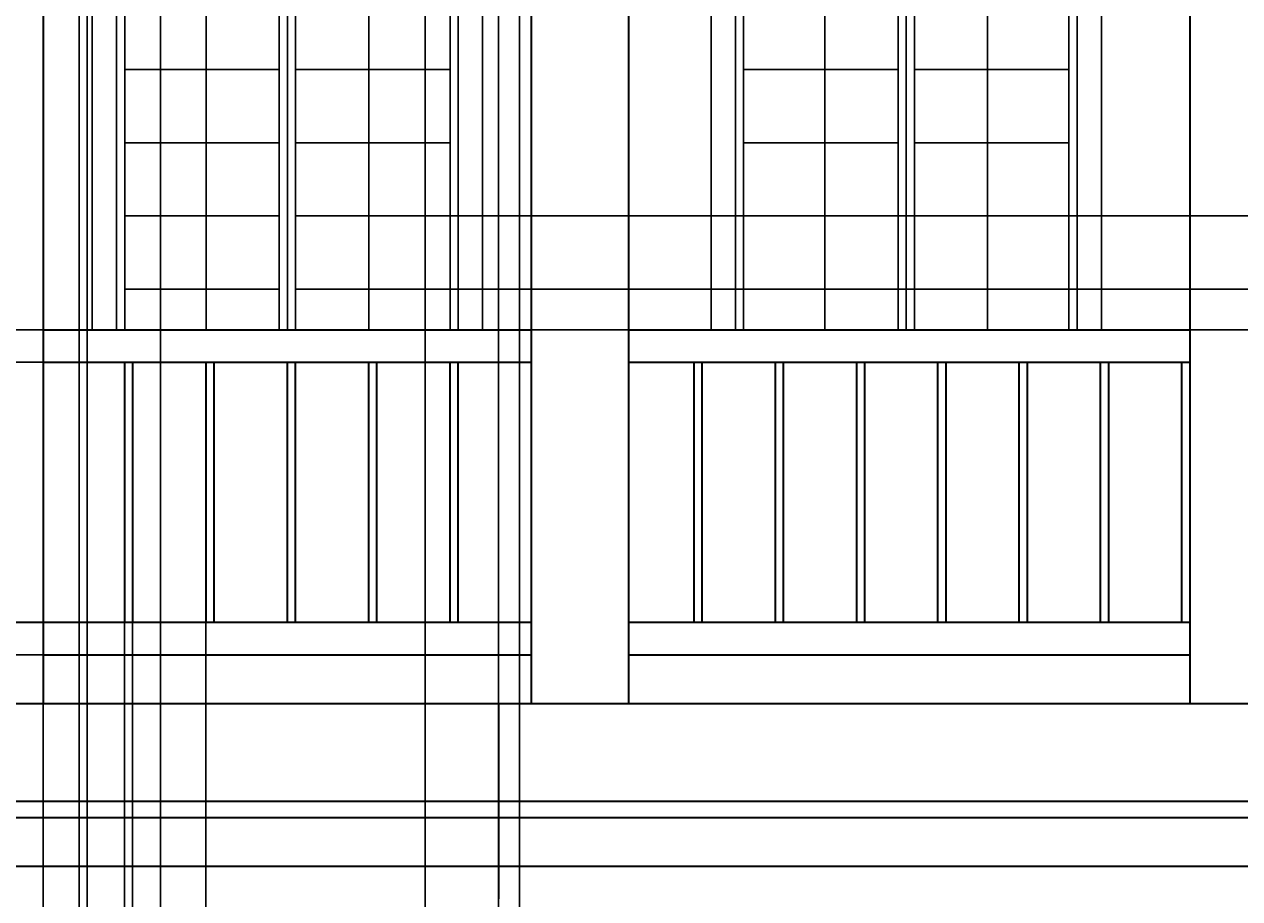
# Model space of a CAD drawing. Units: inches. Extents: x 2154 to 2740, y 571 to 1084.
# Tile 3 of 13: x 2235 to 2384, y 754 to 861. Entities that reach past the tile are written whole.
import ezdxf

# ---------------------------------------------------------------- set-up
doc = ezdxf.new("R2010")
doc.units = ezdxf.units.IN
for name, color, linetype, lineweight in [('A-ANNO-DIMS', 2, 'Continuous', 18), ('A-ELEV', 7, 'Continuous', 35), ('A-GLAZ', 4, 'Continuous', 25)]:
    doc.layers.add(name, color=color, linetype=linetype, lineweight=lineweight)
doc.styles.get("Standard").update_dxf_attribs({"font": 'arial.ttf'})
doc.dimstyles.get("Standard").update_dxf_attribs({"dimtxt": 0.18, "dimasz": 0.18, "dimexe": 0.18, "dimexo": 0.0625, "dimgap": 0.09, "dimtad": 0, "dimtih": 1, "dimtoh": 1, "dimdec": 4, "dimzin": 0, "dimdsep": 46, "dimtxsty": 'Standard', "dimcen": 0.09, "dimadec": 0, "dimazin": 0, "dimtfac": 1, "dimtdec": 4, "dimtofl": 0, "dimtmove": 0, "dimatfit": 3, "dimfxl": 1, "dimtolj": 1, "dimtzin": 0, "dimarcsym": 0})

# ---------------------------------------------------------------- blocks, each defined once
blk = doc.blocks.new('WIN-ELEV-1200')
for p, q in [((0, 50), (48, 50)), ((0, 0), (0, 50)), ((48, 0), (48, 50)), ((3, 0), (3, 47)), ((3, 47), (45, 47)), ((45, 0), (45, 47)), ((4, 46), (44, 46)), ((4, 0), (4, 46)), ((14, 0), (14, 46)), ((23, 0), (23, 46)), ((24, 0), (24, 46)), ((25, 0), (25, 46)), ((34, 0), (34, 46)), ((44, 0), (44, 46)), ((4, 41), (23, 41)), ((25, 41), (44, 41)), ((4, 32), (23, 32)), ((25, 32), (44, 32)), ((4, 23), (23, 23)), ((25, 23), (44, 23)), ((4, 14), (23, 14)), ((25, 14), (44, 14)), ((4, 5), (23, 5)), ((25, 5), (44, 5))]:
    blk.add_line(p, q)
blk = doc.blocks.new('*D10')
at = {"layer": 'A-ANNO-DIMS', "color": 0, "lineweight": -2, "transparency": 16777216}
for p, q in [((2447.14, 1057.01), (2154.18, 1057.01)), ((2154.36, 1056.83), (2154.36, 827.45)), ((2154.36, 597.71), (2154.36, 827.09)), ((2181.14, 597.53), (2154.18, 597.53))]:
    blk.add_line(p, q, dxfattribs=at)
at = {"layer": 'A-ANNO-DIMS', "color": 0, "transparency": 16777216}
for points in [[(2154.33, 1056.83), (2154.39, 1056.83), (2154.36, 1057.01)], [(2154.33, 597.71), (2154.39, 597.71), (2154.36, 597.53)]]:
    blk.add_solid(points, dxfattribs=at)
at = {"layer": 'Defpoints', "color": 0, "transparency": 16777216}
for p in [(2154.36, 1057.01), (2447.21, 1057.01), (2181.21, 597.53)]:
    blk.add_point(p, dxfattribs=at)
at = {"layer": 'A-ANNO-DIMS', "color": 0, "transparency": 16777216, "insert": (2154.36, 827.27), "char_height": 0.18, "attachment_point": 5}
blk.add_mtext('\\A1;459.5', dxfattribs=at)
blk = doc.blocks.new('*D30')
at = {"layer": 'A-ANNO-DIMS', "color": 0, "lineweight": -2, "transparency": 16777216}
for p, q in [((2657.14, 823.53), (2154.18, 823.53)), ((2154.36, 823.35), (2154.36, 800.71)), ((2154.36, 777.71), (2154.36, 800.35)), ((2657.14, 777.53), (2154.18, 777.53))]:
    blk.add_line(p, q, dxfattribs=at)
at = {"layer": 'A-ANNO-DIMS', "color": 0, "transparency": 16777216}
for points in [[(2154.33, 823.35), (2154.39, 823.35), (2154.36, 823.53)], [(2154.33, 777.71), (2154.39, 777.71), (2154.36, 777.53)]]:
    blk.add_solid(points, dxfattribs=at)
at = {"layer": 'Defpoints', "color": 0, "transparency": 16777216}
for p in [(2154.36, 823.53), (2657.21, 823.53), (2657.21, 777.53)]:
    blk.add_point(p, dxfattribs=at)
at = {"layer": 'A-ANNO-DIMS', "color": 0, "transparency": 16777216, "insert": (2154.36, 800.53), "char_height": 0.18, "attachment_point": 5}
blk.add_mtext('\\A1;46', dxfattribs=at)
blk = doc.blocks.new('*D33')
at = {"layer": 'A-ANNO-DIMS', "color": 0, "lineweight": -2, "transparency": 16777216}
for p, q in [((2412.64, 873.53), (2154.18, 873.53)), ((2154.36, 873.35), (2154.36, 848.71)), ((2154.36, 823.71), (2154.36, 848.35)), ((2412.64, 823.53), (2154.18, 823.53))]:
    blk.add_line(p, q, dxfattribs=at)
at = {"layer": 'A-ANNO-DIMS', "color": 0, "transparency": 16777216}
for points in [[(2154.33, 873.35), (2154.39, 873.35), (2154.36, 873.53)], [(2154.33, 823.71), (2154.39, 823.71), (2154.36, 823.53)]]:
    blk.add_solid(points, dxfattribs=at)
at = {"layer": 'Defpoints', "color": 0, "transparency": 16777216}
for p in [(2154.36, 873.53), (2412.71, 873.53), (2412.71, 823.53)]:
    blk.add_point(p, dxfattribs=at)
at = {"layer": 'A-ANNO-DIMS', "color": 0, "transparency": 16777216, "insert": (2154.36, 848.53), "char_height": 0.18, "attachment_point": 5}
blk.add_mtext('\\A1;50', dxfattribs=at)
blk = doc.blocks.new('*D39')
at = {"layer": 'A-ANNO-DIMS', "color": 0, "lineweight": -2, "transparency": 16777216}
for p, q in [((2183.21, 979.47), (2183.21, 570.5)), ((2417.21, 970.47), (2417.21, 570.5)), ((2183.39, 570.68), (2299.92, 570.68)), ((2417.03, 570.68), (2300.5, 570.68))]:
    blk.add_line(p, q, dxfattribs=at)
at = {"layer": 'A-ANNO-DIMS', "color": 0, "transparency": 16777216}
for points in [[(2183.39, 570.71), (2183.39, 570.65), (2183.21, 570.68)], [(2417.03, 570.71), (2417.03, 570.65), (2417.21, 570.68)]]:
    blk.add_solid(points, dxfattribs=at)
at = {"layer": 'Defpoints', "color": 0, "transparency": 16777216}
for p in [(2183.21, 979.53), (2417.21, 970.53), (2417.21, 570.68)]:
    blk.add_point(p, dxfattribs=at)
at = {"layer": 'A-ANNO-DIMS', "color": 0, "transparency": 16777216, "insert": (2300.21, 570.68), "char_height": 0.18, "attachment_point": 5}
blk.add_mtext('\\A1;234', dxfattribs=at)
blk = doc.blocks.new('*D52')
at = {"layer": 'A-ANNO-DIMS', "color": 0, "lineweight": -2, "transparency": 16777216}
for p, q in [((2284.21, 903.47), (2284.21, 570.5)), ((2293.21, 903.47), (2293.21, 570.5)), ((2284.39, 570.68), (2288.56, 570.68)), ((2293.03, 570.68), (2288.86, 570.68))]:
    blk.add_line(p, q, dxfattribs=at)
at = {"layer": 'A-ANNO-DIMS', "color": 0, "transparency": 16777216}
for points in [[(2284.39, 570.71), (2284.39, 570.65), (2284.21, 570.68)], [(2293.03, 570.71), (2293.03, 570.65), (2293.21, 570.68)]]:
    blk.add_solid(points, dxfattribs=at)
at = {"layer": 'Defpoints', "color": 0, "transparency": 16777216}
for p in [(2284.21, 903.53), (2293.21, 903.53), (2293.21, 570.68)]:
    blk.add_point(p, dxfattribs=at)
at = {"layer": 'A-ANNO-DIMS', "color": 0, "transparency": 16777216, "insert": (2288.71, 570.68), "char_height": 0.18, "attachment_point": 5}
blk.add_mtext('\\A1;9', dxfattribs=at)
blk = doc.blocks.new('*D56')
at = {"layer": 'A-ANNO-DIMS', "color": 0, "lineweight": -2, "transparency": 16777216}
for p, q in [((2293.21, 915.47), (2293.21, 570.5)), ((2295.77, 915.97), (2295.77, 570.5)), ((2293.39, 570.68), (2294.16, 570.68)), ((2295.59, 570.68), (2294.81, 570.68))]:
    blk.add_line(p, q, dxfattribs=at)
at = {"layer": 'A-ANNO-DIMS', "color": 0, "transparency": 16777216}
for points in [[(2293.39, 570.71), (2293.39, 570.65), (2293.21, 570.68)], [(2295.59, 570.71), (2295.59, 570.65), (2295.77, 570.68)]]:
    blk.add_solid(points, dxfattribs=at)
at = {"layer": 'Defpoints', "color": 0, "transparency": 16777216}
for p in [(2293.21, 915.53), (2295.77, 916.03), (2295.77, 570.68)]:
    blk.add_point(p, dxfattribs=at)
at = {"layer": 'A-ANNO-DIMS', "color": 0, "transparency": 16777216, "insert": (2294.49, 570.68), "char_height": 0.18, "attachment_point": 5}
blk.add_mtext('\\A1;2.56', dxfattribs=at)
blk = doc.blocks.new('*D65')
at = {"layer": 'A-ANNO-DIMS', "color": 0, "lineweight": -2, "transparency": 16777216}
for p, q in [((2225.21, 777.59), (2225.21, 1084.04)), ((2225.39, 1083.86), (2231, 1083.86)), ((2237.03, 1083.86), (2231.42, 1083.86)), ((2237.21, 777.59), (2237.21, 1084.04))]:
    blk.add_line(p, q, dxfattribs=at)
at = {"layer": 'A-ANNO-DIMS', "color": 0, "transparency": 16777216}
for points in [[(2225.39, 1083.89), (2225.39, 1083.83), (2225.21, 1083.86)], [(2237.03, 1083.89), (2237.03, 1083.83), (2237.21, 1083.86)]]:
    blk.add_solid(points, dxfattribs=at)
at = {"layer": 'Defpoints', "color": 0, "transparency": 16777216}
for p in [(2237.21, 1083.86), (2225.21, 777.53), (2237.21, 777.53)]:
    blk.add_point(p, dxfattribs=at)
at = {"layer": 'A-ANNO-DIMS', "color": 0, "transparency": 16777216, "insert": (2231.21, 1083.86), "char_height": 0.18, "attachment_point": 5}
blk.add_mtext('\\A1;12', dxfattribs=at)
blk = doc.blocks.new('*D110')
at = {"layer": 'A-ANNO-DIMS', "color": 0, "lineweight": -2, "transparency": 16777216}
for p, q in [((2237.21, 823.59), (2237.21, 1084.04)), ((2237.39, 1083.86), (2239.91, 1083.86)), ((2243.08, 1083.86), (2240.56, 1083.86)), ((2243.26, 823.59), (2243.26, 1084.04))]:
    blk.add_line(p, q, dxfattribs=at)
at = {"layer": 'A-ANNO-DIMS', "color": 0, "transparency": 16777216}
for points in [[(2237.39, 1083.89), (2237.39, 1083.83), (2237.21, 1083.86)], [(2243.08, 1083.89), (2243.08, 1083.83), (2243.26, 1083.86)]]:
    blk.add_solid(points, dxfattribs=at)
at = {"layer": 'Defpoints', "color": 0, "transparency": 16777216}
for p in [(2243.26, 1083.86), (2237.21, 823.53), (2243.26, 823.53)]:
    blk.add_point(p, dxfattribs=at)
at = {"layer": 'A-ANNO-DIMS', "color": 0, "transparency": 16777216, "insert": (2240.23, 1083.86), "char_height": 0.18, "attachment_point": 5}
blk.add_mtext('\\A1;6.05', dxfattribs=at)
blk = doc.blocks.new('*D119')
at = {"layer": 'A-ANNO-DIMS', "color": 0, "lineweight": -2, "transparency": 16777216}
for p, q in [((2287.32, 828.53), (2740.24, 828.53)), ((2740.06, 828.35), (2740.06, 826.21)), ((2740.06, 823.71), (2740.06, 825.85)), ((2287.32, 823.53), (2740.24, 823.53))]:
    blk.add_line(p, q, dxfattribs=at)
at = {"layer": 'A-ANNO-DIMS', "color": 0, "transparency": 16777216}
for points in [[(2740.03, 828.35), (2740.09, 828.35), (2740.06, 828.53)], [(2740.03, 823.71), (2740.09, 823.71), (2740.06, 823.53)]]:
    blk.add_solid(points, dxfattribs=at)
at = {"layer": 'Defpoints', "color": 0, "transparency": 16777216}
for p in [(2287.26, 828.53), (2740.06, 828.53), (2287.26, 823.53)]:
    blk.add_point(p, dxfattribs=at)
at = {"layer": 'A-ANNO-DIMS', "color": 0, "transparency": 16777216, "insert": (2740.06, 826.03), "char_height": 0.18, "attachment_point": 5}
blk.add_mtext('\\A1;5', dxfattribs=at)
blk = doc.blocks.new('*D120')
at = {"layer": 'A-ANNO-DIMS', "color": 0, "lineweight": -2, "transparency": 16777216}
for p, q in [((2287.32, 837.53), (2740.24, 837.53)), ((2740.06, 837.35), (2740.06, 833.21)), ((2740.06, 828.71), (2740.06, 832.85)), ((2287.32, 828.53), (2740.24, 828.53))]:
    blk.add_line(p, q, dxfattribs=at)
at = {"layer": 'A-ANNO-DIMS', "color": 0, "transparency": 16777216}
for points in [[(2740.03, 837.35), (2740.09, 837.35), (2740.06, 837.53)], [(2740.03, 828.71), (2740.09, 828.71), (2740.06, 828.53)]]:
    blk.add_solid(points, dxfattribs=at)
at = {"layer": 'Defpoints', "color": 0, "transparency": 16777216}
for p in [(2287.26, 837.53), (2740.06, 837.53), (2287.26, 828.53)]:
    blk.add_point(p, dxfattribs=at)
at = {"layer": 'A-ANNO-DIMS', "color": 0, "transparency": 16777216, "insert": (2740.06, 833.03), "char_height": 0.18, "attachment_point": 5}
blk.add_mtext('\\A1;9', dxfattribs=at)
blk = doc.blocks.new('*D122')
at = {"layer": 'A-ANNO-DIMS', "color": 0, "lineweight": -2, "transparency": 16777216}
for p, q in [((2237.14, 783.53), (2154.18, 783.53)), ((2154.36, 783.35), (2154.36, 780.71)), ((2154.36, 777.71), (2154.36, 780.35)), ((2237.14, 777.53), (2154.18, 777.53))]:
    blk.add_line(p, q, dxfattribs=at)
at = {"layer": 'A-ANNO-DIMS', "color": 0, "transparency": 16777216}
for points in [[(2154.33, 783.35), (2154.39, 783.35), (2154.36, 783.53)], [(2154.33, 777.71), (2154.39, 777.71), (2154.36, 777.53)]]:
    blk.add_solid(points, dxfattribs=at)
at = {"layer": 'Defpoints', "color": 0, "transparency": 16777216}
for p in [(2154.36, 783.53), (2237.21, 783.53), (2237.21, 777.53)]:
    blk.add_point(p, dxfattribs=at)
at = {"layer": 'A-ANNO-DIMS', "color": 0, "transparency": 16777216, "insert": (2154.36, 780.53), "char_height": 0.18, "attachment_point": 5}
blk.add_mtext('\\A1;6', dxfattribs=at)
blk = doc.blocks.new('*D123')
at = {"layer": 'A-ANNO-DIMS', "color": 0, "lineweight": -2, "transparency": 16777216}
for p, q in [((2237.144199, 787.532069), (2154.176699, 787.532069)), ((2154.356699, 787.352069), (2154.356699, 785.712069)), ((2154.356699, 783.712069), (2154.356699, 785.352069)), ((2237.144199, 783.532069), (2154.176699, 783.532069))]:
    blk.add_line(p, q, dxfattribs=at)
at = {"layer": 'A-ANNO-DIMS', "color": 0, "transparency": 16777216}
for points in [[(2154.326699, 787.352069), (2154.386699, 787.352069), (2154.356699, 787.532069)], [(2154.326699, 783.712069), (2154.386699, 783.712069), (2154.356699, 783.532069)]]:
    blk.add_solid(points, dxfattribs=at)
at = {"layer": 'Defpoints', "color": 0, "transparency": 16777216}
for p in [(2154.356699, 787.532069), (2237.206699, 787.532069), (2237.206699, 783.532069)]:
    blk.add_point(p, dxfattribs=at)
at = {"layer": 'A-ANNO-DIMS', "color": 0, "transparency": 16777216, "insert": (2154.356699, 785.532069), "char_height": 0.18, "attachment_point": 5}
blk.add_mtext('\\A1;4', dxfattribs=at)
blk = doc.blocks.new('*D124')
at = {"layer": 'A-ANNO-DIMS', "color": 0, "lineweight": -2, "transparency": 16777216}
for p, q in [((2237.14, 819.53), (2154.18, 819.53)), ((2154.36, 819.35), (2154.36, 803.71)), ((2154.36, 787.71), (2154.36, 803.35)), ((2237.14, 787.53), (2154.18, 787.53))]:
    blk.add_line(p, q, dxfattribs=at)
at = {"layer": 'A-ANNO-DIMS', "color": 0, "transparency": 16777216}
for points in [[(2154.33, 819.35), (2154.39, 819.35), (2154.36, 819.53)], [(2154.33, 787.71), (2154.39, 787.71), (2154.36, 787.53)]]:
    blk.add_solid(points, dxfattribs=at)
at = {"layer": 'Defpoints', "color": 0, "transparency": 16777216}
for p in [(2154.36, 819.53), (2237.21, 819.53), (2237.21, 787.53)]:
    blk.add_point(p, dxfattribs=at)
at = {"layer": 'A-ANNO-DIMS', "color": 0, "transparency": 16777216, "insert": (2154.36, 803.53), "char_height": 0.18, "attachment_point": 5}
blk.add_mtext('\\A1;32', dxfattribs=at)
blk = doc.blocks.new('*D125')
at = {"layer": 'A-ANNO-DIMS', "color": 0, "lineweight": -2, "transparency": 16777216}
for p, q in [((2237.144199, 823.532069), (2154.176699, 823.532069)), ((2154.356699, 823.352069), (2154.356699, 821.712069)), ((2154.356699, 819.712069), (2154.356699, 821.352069)), ((2237.144199, 819.532069), (2154.176699, 819.532069))]:
    blk.add_line(p, q, dxfattribs=at)
at = {"layer": 'A-ANNO-DIMS', "color": 0, "transparency": 16777216}
for points in [[(2154.326699, 823.352069), (2154.386699, 823.352069), (2154.356699, 823.532069)], [(2154.326699, 819.712069), (2154.386699, 819.712069), (2154.356699, 819.532069)]]:
    blk.add_solid(points, dxfattribs=at)
at = {"layer": 'Defpoints', "color": 0, "transparency": 16777216}
for p in [(2154.356699, 823.532069), (2237.206699, 823.532069), (2237.206699, 819.532069)]:
    blk.add_point(p, dxfattribs=at)
at = {"layer": 'A-ANNO-DIMS', "color": 0, "transparency": 16777216, "insert": (2154.356699, 821.532069), "char_height": 0.18, "attachment_point": 5}
blk.add_mtext('\\A1;4', dxfattribs=at)
blk = doc.blocks.new('*D126')
at = {"layer": 'A-ANNO-DIMS', "color": 0, "lineweight": -2, "transparency": 16777216}
for p, q in [((2237.21, 787.47), (2237.21, 570.5)), ((2247.21, 787.47), (2247.21, 570.5)), ((2237.39, 570.68), (2242, 570.68)), ((2247.03, 570.68), (2242.42, 570.68))]:
    blk.add_line(p, q, dxfattribs=at)
at = {"layer": 'A-ANNO-DIMS', "color": 0, "transparency": 16777216}
for points in [[(2237.39, 570.71), (2237.39, 570.65), (2237.21, 570.68)], [(2247.03, 570.71), (2247.03, 570.65), (2247.21, 570.68)]]:
    blk.add_solid(points, dxfattribs=at)
at = {"layer": 'Defpoints', "color": 0, "transparency": 16777216}
for p in [(2237.21, 787.53), (2247.21, 787.53), (2247.21, 570.68)]:
    blk.add_point(p, dxfattribs=at)
at = {"layer": 'A-ANNO-DIMS', "color": 0, "transparency": 16777216, "insert": (2242.21, 570.68), "char_height": 0.18, "attachment_point": 5}
blk.add_mtext('\\A1;10', dxfattribs=at)
blk = doc.blocks.new('*D127')
at = {"layer": 'A-ANNO-DIMS', "color": 0, "lineweight": -2, "transparency": 16777216}
for p, q in [((2247.21, 787.47), (2247.21, 570.5)), ((2248.21, 787.47), (2248.21, 570.5)), ((2247.39, 570.68), (2247.58, 570.68)), ((2248.03, 570.68), (2247.83, 570.68))]:
    blk.add_line(p, q, dxfattribs=at)
at = {"layer": 'A-ANNO-DIMS', "color": 0, "transparency": 16777216}
for points in [[(2247.39, 570.71), (2247.39, 570.65), (2247.21, 570.68)], [(2248.03, 570.71), (2248.03, 570.65), (2248.21, 570.68)]]:
    blk.add_solid(points, dxfattribs=at)
at = {"layer": 'Defpoints', "color": 0, "transparency": 16777216}
for p in [(2247.21, 787.53), (2248.21, 787.53), (2248.21, 570.68)]:
    blk.add_point(p, dxfattribs=at)
at = {"layer": 'A-ANNO-DIMS', "color": 0, "transparency": 16777216, "insert": (2247.71, 570.68), "char_height": 0.18, "attachment_point": 5}
blk.add_mtext('\\A1;1', dxfattribs=at)
blk = doc.blocks.new('*D128')
at = {"layer": 'A-ANNO-DIMS', "color": 0, "lineweight": -2, "transparency": 16777216}
for p, q in [((2248.21, 787.47), (2248.21, 570.5)), ((2257.21, 787.47), (2257.21, 570.5)), ((2248.39, 570.68), (2252.56, 570.68)), ((2257.03, 570.68), (2252.86, 570.68))]:
    blk.add_line(p, q, dxfattribs=at)
at = {"layer": 'A-ANNO-DIMS', "color": 0, "transparency": 16777216}
for points in [[(2248.39, 570.71), (2248.39, 570.65), (2248.21, 570.68)], [(2257.03, 570.71), (2257.03, 570.65), (2257.21, 570.68)]]:
    blk.add_solid(points, dxfattribs=at)
at = {"layer": 'Defpoints', "color": 0, "transparency": 16777216}
for p in [(2248.21, 787.53), (2257.21, 787.53), (2257.21, 570.68)]:
    blk.add_point(p, dxfattribs=at)
at = {"layer": 'A-ANNO-DIMS', "color": 0, "transparency": 16777216, "insert": (2252.71, 570.68), "char_height": 0.18, "attachment_point": 5}
blk.add_mtext('\\A1;9', dxfattribs=at)
blk = doc.blocks.new('*D136')
at = {"layer": 'A-ANNO-DIMS', "color": 0, "lineweight": -2, "transparency": 16777216}
for p, q in [((2241.65, 648.59), (2241.65, 1084.04)), ((2241.83, 1083.86), (2242.03, 1083.86)), ((2242.47, 1083.86), (2242.28, 1083.86)), ((2242.65, 648.59), (2242.65, 1084.04))]:
    blk.add_line(p, q, dxfattribs=at)
at = {"layer": 'A-ANNO-DIMS', "color": 0, "transparency": 16777216}
for points in [[(2241.83, 1083.89), (2241.83, 1083.83), (2241.65, 1083.86)], [(2242.47, 1083.89), (2242.47, 1083.83), (2242.65, 1083.86)]]:
    blk.add_solid(points, dxfattribs=at)
at = {"layer": 'Defpoints', "color": 0, "transparency": 16777216}
for p in [(2242.65, 1083.86), (2241.65, 648.53), (2242.65, 648.53)]:
    blk.add_point(p, dxfattribs=at)
at = {"layer": 'A-ANNO-DIMS', "color": 0, "transparency": 16777216, "insert": (2242.15, 1083.86), "char_height": 0.18, "attachment_point": 5}
blk.add_mtext('\\A1;1', dxfattribs=at)
blk = doc.blocks.new('*D137')
at = {"layer": 'A-ANNO-DIMS', "color": 0, "lineweight": -2, "transparency": 16777216}
for p, q in [((2242.65, 648.59), (2242.65, 1084.04)), ((2242.83, 1083.86), (2247, 1083.86)), ((2251.47, 1083.86), (2247.3, 1083.86)), ((2251.65, 648.59), (2251.65, 1084.04))]:
    blk.add_line(p, q, dxfattribs=at)
at = {"layer": 'A-ANNO-DIMS', "color": 0, "transparency": 16777216}
for points in [[(2242.83, 1083.89), (2242.83, 1083.83), (2242.65, 1083.86)], [(2251.47, 1083.89), (2251.47, 1083.83), (2251.65, 1083.86)]]:
    blk.add_solid(points, dxfattribs=at)
at = {"layer": 'Defpoints', "color": 0, "transparency": 16777216}
for p in [(2251.65, 1083.86), (2242.65, 648.53), (2251.65, 648.53)]:
    blk.add_point(p, dxfattribs=at)
at = {"layer": 'A-ANNO-DIMS', "color": 0, "transparency": 16777216, "insert": (2247.15, 1083.86), "char_height": 0.18, "attachment_point": 5}
blk.add_mtext('\\A1;9', dxfattribs=at)

msp = doc.modelspace()

# ---------------------------------------------------------------- linework, layer by layer
at = {"layer": 'A-ELEV'}
for p, q in [((2237.2067, 903.5321), (2237.2067, 777.5321)), ((2297.2067, 903.5321), (2297.2067, 777.5321)), ((2309.2067, 903.5321), (2309.2067, 777.5321)), ((2378.2067, 903.5321), (2378.2067, 777.5321)), ((2237.2067, 823.5321), (2297.2067, 823.5321)), ((2309.2067, 823.5321), (2378.2067, 823.5321)), ((2237.2067, 819.5321), (2297.2067, 819.5321)), ((2247.2067, 819.5321), (2247.2067, 787.5321)), ((2248.2067, 819.5321), (2248.2067, 787.5321)), ((2257.2067, 819.5321), (2257.2067, 787.5321)), ((2258.2067, 819.5321), (2258.2067, 787.5321)), ((2267.2067, 819.5321), (2267.2067, 787.5321)), ((2268.2067, 819.5321), (2268.2067, 787.5321)), ((2277.2067, 819.5321), (2277.2067, 787.5321)), ((2278.2067, 819.5321), (2278.2067, 787.5321)), ((2287.2067, 819.5321), (2287.2067, 787.5321)), ((2288.2067, 819.5321), (2288.2067, 787.5321)), ((2297.2067, 819.5321), (2297.2067, 787.5321)), ((2309.2067, 819.5321), (2378.2067, 819.5321)), ((2317.2067, 819.5321), (2317.2067, 787.5321)), ((2318.2067, 819.5321), (2318.2067, 787.5321)), ((2327.2067, 819.5321), (2327.2067, 787.5321)), ((2328.2067, 819.5321), (2328.2067, 787.5321)), ((2337.2067, 819.5321), (2337.2067, 787.5321)), ((2338.2067, 819.5321), (2338.2067, 787.5321)), ((2347.2067, 819.5321), (2347.2067, 787.5321)), ((2348.2067, 819.5321), (2348.2067, 787.5321)), ((2357.2067, 819.5321), (2357.2067, 787.5321)), ((2358.2067, 819.5321), (2358.2067, 787.5321)), ((2367.2067, 819.5321), (2367.2067, 787.5321)), ((2368.2067, 819.5321), (2368.2067, 787.5321)), ((2377.2067, 819.5321), (2377.2067, 787.5321)), ((2378.2067, 819.5321), (2378.2067, 787.5321)), ((2237.2067, 787.5321), (2297.2067, 787.5321)), ((2309.2067, 787.5321), (2378.2067, 787.5321)), ((2237.2067, 783.5321), (2297.2067, 783.5321)), ((2309.2067, 783.5321), (2378.2067, 783.5321)), ((2219.2067, 777.5321), (2675.2067, 777.5321)), ((2293.2067, 777.5321), (2293.2067, 753.5321)), ((2221.2067, 765.5321), (2673.2067, 765.5321)), ((2221.2067, 763.5321), (2673.2067, 763.5321)), ((2183.2067, 757.5321), (2711.2067, 757.5321))]:
    msp.add_line(p, q, dxfattribs=at)

# ---------------------------------------------------------------- block references
at = {"layer": 'A-GLAZ'}
for p in [(2243.2571, 823.532), (2319.3479, 823.532)]:
    msp.add_blockref('WIN-ELEV-1200', p, dxfattribs=at)

# ---------------------------------------------------------------- dimensions: what is measured, and where the dimension line sits
at = {"layer": 'A-ANNO-DIMS'}
for base, p1, p2, override, picture, middle in [((2237.2067, 1083.8553), (2225.2067, 777.5321), (2237.2067, 777.5321), {"dimdec": 0, "dimlfac": 1, "dimrnd": 0, "dimzin": 0, "dimdsep": 46, "dimlunit": 2}, '*D65', (2231.2067, 1083.8553)), ((2243.2568, 1083.8553), (2237.2067, 823.5321), (2243.2568, 823.5321), {"dimdec": 2, "dimlfac": 1, "dimrnd": 0, "dimzin": 0, "dimdsep": 46, "dimlunit": 2}, '*D110', (2240.2317, 1083.8553)), ((2242.6527, 1083.8553), (2241.6527, 648.5321), (2242.6527, 648.5321), {"dimdec": 0, "dimlfac": 1, "dimrnd": 0, "dimzin": 0, "dimdsep": 46, "dimlunit": 2}, '*D136', (2242.1527, 1083.8553)), ((2251.6527, 1083.8553), (2242.6527, 648.5321), (2251.6527, 648.5321), {"dimdec": 0, "dimlfac": 1, "dimrnd": 0, "dimzin": 0, "dimdsep": 46, "dimlunit": 2}, '*D137', (2247.1527, 1083.8553)), ((2417.2067, 570.6821), (2183.2067, 979.5321), (2417.2067, 970.5321), {"dimdec": 0, "dimlfac": 1, "dimrnd": 0, "dimzin": 0, "dimdsep": 46, "dimlunit": 2}, '*D39', (2300.2067, 570.6821)), ((2295.7714, 570.6821), (2293.2067, 915.5321), (2295.7714, 916.028), {"dimdec": 2, "dimlfac": 1, "dimrnd": 0, "dimzin": 0, "dimdsep": 46, "dimlunit": 2}, '*D56', (2294.4891, 570.6821)), ((2293.2067, 570.6821), (2284.2067, 903.5321), (2293.2067, 903.5321), {"dimdec": 0, "dimlfac": 1, "dimrnd": 0, "dimzin": 0, "dimdsep": 46, "dimlunit": 2}, '*D52', (2288.7067, 570.6821)), ((2247.2067, 570.6821), (2237.2067, 787.5321), (2247.2067, 787.5321), {"dimdec": 0, "dimlfac": 1, "dimrnd": 0, "dimzin": 0, "dimdsep": 46, "dimlunit": 2}, '*D126', (2242.2067, 570.6821)), ((2248.2067, 570.6821), (2247.2067, 787.5321), (2248.2067, 787.5321), {"dimdec": 0, "dimlfac": 1, "dimrnd": 0, "dimzin": 0, "dimdsep": 46, "dimlunit": 2}, '*D127', (2247.7067, 570.6821)), ((2257.2067, 570.6821), (2248.2067, 787.5321), (2257.2067, 787.5321), {"dimdec": 0, "dimlfac": 1, "dimrnd": 0, "dimzin": 0, "dimdsep": 46, "dimlunit": 2}, '*D128', (2252.7067, 570.6821))]:
    dim = msp.add_linear_dim(base=base, p1=p1, p2=p2, dimstyle='Standard', override=override, dxfattribs=at)
    dim.commit()
    dim.dimension.update_dxf_attribs({"geometry": picture, "text_midpoint": middle})
for base, p1, p2, override, picture, middle in [((2154.3567, 1057.0053), (2181.2067, 597.5321), (2447.2067, 1057.0053), {"dimdec": 1, "dimlfac": 1, "dimrnd": 0, "dimzin": 0, "dimdsep": 46, "dimlunit": 2}, '*D10', (2154.3567, 827.2687)), ((2154.3567, 873.5321), (2412.7067, 823.5321), (2412.7067, 873.5321), {"dimdec": 0, "dimlfac": 1, "dimrnd": 0, "dimzin": 0, "dimdsep": 46, "dimlunit": 2}, '*D33', (2154.3567, 848.5321)), ((2740.0567, 837.5321), (2287.2568, 828.5321), (2287.2568, 837.5321), {"dimdec": 0, "dimlfac": 1, "dimrnd": 0, "dimzin": 0, "dimdsep": 46, "dimlunit": 2}, '*D120', (2740.0567, 833.0321)), ((2740.0567, 828.5321), (2287.2568, 823.5321), (2287.2568, 828.5321), {"dimdec": 0, "dimlfac": 1, "dimrnd": 0, "dimzin": 0, "dimdsep": 46, "dimlunit": 2}, '*D119', (2740.0567, 826.0321)), ((2154.3567, 823.5321), (2657.2067, 777.5321), (2657.2067, 823.5321), {"dimdec": 0, "dimlfac": 1, "dimrnd": 0, "dimzin": 0, "dimdsep": 46, "dimlunit": 2}, '*D30', (2154.3567, 800.5321)), ((2154.3567, 823.5321), (2237.2067, 819.5321), (2237.2067, 823.5321), {"dimdec": 0, "dimlfac": 1, "dimrnd": 0, "dimzin": 0, "dimdsep": 46, "dimlunit": 2}, '*D125', (2154.3567, 821.5321)), ((2154.3567, 819.5321), (2237.2067, 787.5321), (2237.2067, 819.5321), {"dimdec": 0, "dimlfac": 1, "dimrnd": 0, "dimzin": 0, "dimdsep": 46, "dimlunit": 2}, '*D124', (2154.3567, 803.5321)), ((2154.3567, 787.5321), (2237.2067, 783.5321), (2237.2067, 787.5321), {"dimdec": 0, "dimlfac": 1, "dimrnd": 0, "dimzin": 0, "dimdsep": 46, "dimlunit": 2}, '*D123', (2154.3567, 785.5321)), ((2154.3567, 783.5321), (2237.2067, 777.5321), (2237.2067, 783.5321), {"dimdec": 0, "dimlfac": 1, "dimrnd": 0, "dimzin": 0, "dimdsep": 46, "dimlunit": 2}, '*D122', (2154.3567, 780.5321))]:
    dim = msp.add_linear_dim(base=base, p1=p1, p2=p2, angle=90, dimstyle='Standard', override=override, dxfattribs=at)
    dim.commit()
    dim.dimension.update_dxf_attribs({"geometry": picture, "text_midpoint": middle})

doc.saveas('drawing.dxf')
